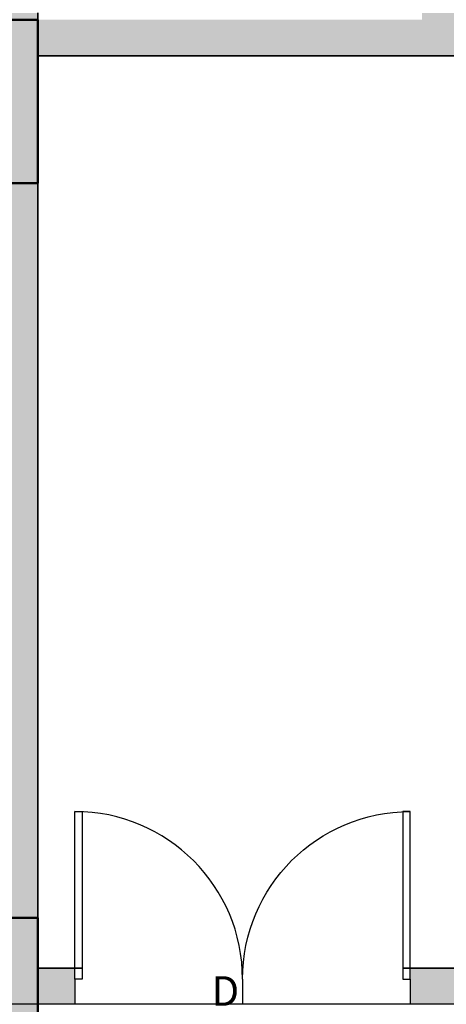
# Model space of a CAD drawing. Units: inches. Extents: x 1998 to 2588, y 1139 to 1977.
# Tile 122 of 134: x 2344 to 2397, y 1637 to 1760. Entities that reach past the tile are written whole.
import ezdxf

# ---------------------------------------------------------------- set-up
doc = ezdxf.new("R2010")
doc.units = ezdxf.units.IN
for name, color, linetype, lineweight in [('A-ANNO-DIMS', 2, 'Continuous', 18), ('A-COLS-PATT', 250, 'Continuous', 13), ('A-DOOR-IDEN', 7, 'Continuous', 18), ('A-WALL-PATT', 252, 'Continuous', 13), ('COLUMN', 10, 'Continuous', 50), ('DOOR', 52, 'Continuous', 25), ('WALL', 200, 'Continuous', 35)]:
    doc.layers.add(name, color=color, linetype=linetype, lineweight=lineweight)
doc.styles.get("Standard").update_dxf_attribs({"font": 'arial.ttf'})
doc.dimstyles.get("Standard").update_dxf_attribs({"dimtxt": 0.18, "dimasz": 0.18, "dimexe": 0.18, "dimexo": 0.0625, "dimgap": 0.09, "dimtad": 0, "dimtih": 1, "dimtoh": 1, "dimdec": 4, "dimzin": 0, "dimdsep": 46, "dimtxsty": 'Standard', "dimcen": 0.09, "dimadec": 0, "dimazin": 0, "dimtfac": 1, "dimtdec": 4, "dimtofl": 0, "dimtmove": 0, "dimatfit": 3, "dimfxl": 1, "dimtolj": 1, "dimtzin": 0, "dimarcsym": 0})

# ---------------------------------------------------------------- blocks, each defined once
blk = doc.blocks.new('*U2')
for p, q in [((0, 0), (0, -6)), ((40, 0), (40, -6))]:
    blk.add_line(p, q)
blk.add_lwpolyline([(0, 0), (0, 40), (1.75, 40), (1.75, 0)], close=True)
blk.add_arc((0, 0), 40, 0, 90)
blk = doc.blocks.new('*D30')
at = {"layer": 'A-ANNO-DIMS', "color": 0, "lineweight": -2, "transparency": 16777216}
for p, q in [((2407.91, 1636.73), (1997.84, 1636.73)), ((1998.02, 1636.55), (1998.02, 1615.91)), ((1998.02, 1594.91), (1998.02, 1615.55)), ((2407.91, 1594.73), (1997.84, 1594.73))]:
    blk.add_line(p, q, dxfattribs=at)
at = {"layer": 'A-ANNO-DIMS', "color": 0, "transparency": 16777216}
for points in [[(1997.99, 1636.55), (1998.05, 1636.55), (1998.02, 1636.73)], [(1997.99, 1594.91), (1998.05, 1594.91), (1998.02, 1594.73)]]:
    blk.add_solid(points, dxfattribs=at)
at = {"layer": 'Defpoints', "color": 0, "transparency": 16777216}
for p in [(1998.02, 1636.73), (2407.97, 1636.73), (2407.97, 1594.73)]:
    blk.add_point(p, dxfattribs=at)
at = {"layer": 'A-ANNO-DIMS', "color": 0, "transparency": 16777216, "insert": (1998.02, 1615.73), "char_height": 0.18, "attachment_point": 5}
blk.add_mtext('\\A1;42', dxfattribs=at)

msp = doc.modelspace()

# ---------------------------------------------------------------- hatches: boundary and pattern name
at = {"layer": 'A-COLS-PATT'}
h = msp.add_hatch(color=256, dxfattribs=at)
h.dxf.hatch_style = 1
h.paths.add_polyline_path([(2099.4125, 1888.7324), (2087.9729, 1888.7324), (2087.9729, 1868.3278), (2099.4125, 1868.3278)])
h.paths.add_polyline_path([(2234.4125, 1888.7324), (2222.9729, 1888.7324), (2222.9729, 1868.3278), (2234.4125, 1868.3278)])
h.paths.add_polyline_path([(2341.4729, 1886.637), (2330.0332, 1886.637), (2330.0332, 1866.2324), (2341.4729, 1866.2324)])
h.paths.add_polyline_path([(2507.8006, 1882.7324), (2487.396, 1882.7324), (2487.396, 1871.2927), (2507.8006, 1871.2927)])
h.paths.add_polyline_path([(2510.9729, 1766.672), (2490.5682, 1766.672), (2490.5682, 1755.2324), (2510.9729, 1755.2324)])
h.paths.add_polyline_path([(2345.9729, 1759.7324), (2334.5332, 1759.7324), (2334.5332, 1739.3278), (2345.9729, 1739.3278)])
h.paths.add_polyline_path([(2234.4125, 1774.3318), (2222.9729, 1774.3318), (2222.9729, 1753.9272), (2234.4125, 1753.9272)])
h.paths.add_polyline_path([(2099.4125, 1775.637), (2087.9729, 1775.637), (2087.9729, 1755.2324), (2099.4125, 1755.2324)])
h.paths.add_polyline_path([(2098.0956, 1593.7241), (2077.691, 1593.7241), (2077.691, 1582.2845), (2098.0956, 1582.2845)])
h.paths.add_polyline_path([(2227.4729, 1604.637), (2216.0332, 1604.637), (2216.0332, 1584.2324), (2227.4729, 1584.2324)])
h.paths.add_polyline_path([(2345.9729, 1647.5211), (2334.5332, 1647.5211), (2334.5332, 1627.1165), (2345.9729, 1627.1165)])
h.paths.add_polyline_path([(2522.3775, 1641.2324), (2501.9729, 1641.2324), (2501.9729, 1629.7927), (2522.3775, 1629.7927)])
h.paths.add_polyline_path([(2522.3775, 1480.7324), (2501.9729, 1480.7324), (2501.9729, 1469.2927), (2522.3775, 1469.2927)])
h.paths.add_polyline_path([(2345.9729, 1488.5616), (2334.5332, 1488.5616), (2334.5332, 1468.1569), (2345.9729, 1468.1569)])
h.paths.add_polyline_path([(2234.4125, 1486.137), (2227.4729, 1486.137), (2227.4729, 1465.7324), (2234.4125, 1465.7324)])
h.paths.add_polyline_path([(2227.4729, 1486.137), (2222.9729, 1486.137), (2222.9729, 1465.7324), (2227.4729, 1465.7324)])
h.paths.add_polyline_path([(2108.3775, 1470.2324), (2087.9729, 1470.2324), (2087.9729, 1458.7927), (2108.3775, 1458.7927)])
h.paths.add_polyline_path([(2096.9729, 1365.5012), (2087.9729, 1365.5012), (2087.9729, 1345.0966), (2096.9729, 1345.0966)])
h.paths.add_polyline_path([(2087.9729, 1365.5012), (2085.5332, 1365.5012), (2085.5332, 1345.0966), (2087.9729, 1345.0966)])
h.paths.add_polyline_path([(2234.4125, 1285.137), (2222.9729, 1285.137), (2222.9729, 1264.7324), (2234.4125, 1264.7324)])
h.paths.add_polyline_path([(2345.9729, 1285.137), (2334.5332, 1285.137), (2334.5332, 1264.7324), (2345.9729, 1264.7324)])
h.paths.add_polyline_path([(2503.1458, 1240.172), (2482.7412, 1240.172), (2482.7412, 1228.7324), (2503.1458, 1228.7324)])
h.paths.add_polyline_path([(2510.9729, 1369.172), (2490.5682, 1369.172), (2490.5682, 1357.7324), (2510.9729, 1357.7324)])
at = {"layer": 'A-WALL-PATT'}
h = msp.add_hatch(color=256, dxfattribs=at)
h.dxf.hatch_style = 1
h.paths.add_polyline_path([(2227.4729, 1911.2324), (2222.9729, 1911.2324), (2222.9729, 1888.7324), (2227.4729, 1888.7324)])
h.paths.add_polyline_path([(2236.4493, 1870.3636), (2236.4493, 1875.2324), (2234.4125, 1875.2324), (2234.4125, 1868.3278), (2227.4729, 1868.3278), (2227.4729, 1866.2324), (2236.4493, 1866.2324)])
h.paths.add_polyline_path([(2330.0332, 1875.2324), (2263.9907, 1875.2324), (2263.9907, 1866.2324), (2330.0332, 1866.2324)])
h.paths.add_polyline_path([(2345.9729, 1906.7324), (2393.9729, 1906.7324), (2393.9729, 1882.7324), (2345.9729, 1882.7324), (2345.9729, 1878.2324), (2393.9729, 1878.2324), (2398.4729, 1878.2324), (2398.4729, 1882.7324), (2398.4729, 1911.2324), (2345.9729, 1911.2324), (2341.4729, 1911.2324), (2341.4729, 1866.2324), (2341.4729, 1790.0412), (2345.9729, 1790.0412), (2345.9729, 1875.2324)])
h.paths.add_polyline_path([(2398.4729, 1878.2324), (2393.9729, 1878.2324), (2393.9729, 1798.2324), (2393.9729, 1793.7324), (2398.4729, 1793.7324)], flags=17)
h.paths.add_polyline_path([(2393.9729, 1798.2324), (2375.7311, 1798.2324, -0.00596797), (2375.7384, 1797.6146), (2375.7384, 1793.7324), (2393.9729, 1793.7324)], flags=17)
h.paths.add_polyline_path([(2349.8569, 1797.6146), (2349.8569, 1798.2324), (2345.9729, 1798.2324), (2345.9729, 1793.7324), (2349.8569, 1793.7324)], flags=17)
h.paths.add_polyline_path([(2398.4729, 1793.7324), (2393.9729, 1793.7324), (2393.9729, 1790.0412), (2398.4729, 1790.0412)], flags=17)
h.paths.add_polyline_path([(2527.4729, 1882.7324), (2507.8006, 1882.7324), (2507.8006, 1878.2324), (2518.4729, 1878.2324), (2518.4729, 1759.7324), (2510.9729, 1759.7324), (2510.9729, 1755.2324), (2527.4729, 1755.2324)])
h.paths.add_polyline_path([(2487.396, 1882.7324), (2398.4729, 1882.7324), (2398.4729, 1878.2324), (2487.396, 1878.2324)])
h.paths.add_polyline_path([(2490.5682, 1759.7324), (2345.9729, 1759.7324), (2345.9729, 1755.2324), (2490.5682, 1755.2324)])
h.paths.add_polyline_path([(2398.4729, 1760.5844), (2398.3914, 1760.5844), (2393.9729, 1760.5844), (2393.9729, 1759.7324), (2398.4729, 1759.7324)])
h.paths.add_polyline_path([(2334.5332, 1759.7324), (2234.4125, 1759.7324), (2234.4125, 1755.2324), (2334.5332, 1755.2324)])
h.paths.add_polyline_path([(2345.9729, 1760.5844), (2341.5543, 1760.5844), (2341.4729, 1760.5844), (2341.4729, 1759.7324), (2345.9729, 1759.7324)])
h.paths.add_polyline_path([(2222.9729, 1759.7324), (2221.7204, 1759.7324), (2221.7204, 1755.2324), (2222.9729, 1755.2324)])
h.paths.add_polyline_path([(2061.4729, 1702.7324), (2059.4729, 1702.7324), (2059.4729, 1584.2324), (2061.4729, 1584.2324)])
h.paths.add_polyline_path([(2061.4729, 1584.2324), (2059.4729, 1584.2324), (2059.4729, 1470.2324), (2061.4729, 1470.2324)])
h.paths.add_polyline_path([(2510.9729, 1469.2927), (2501.9729, 1469.2927), (2501.9729, 1369.172), (2510.9729, 1369.172)])
h.paths.add_polyline_path([(2227.4729, 1369.7324), (2227.4729, 1417.7324), (2221.4126, 1417.7324), (2221.4126, 1413.2324), (2222.9729, 1413.2324), (2222.9729, 1293.2324), (2222.9729, 1285.137), (2227.4729, 1285.137)])
h = msp.add_hatch(color=256, dxfattribs=at)
h.dxf.hatch_style = 1
h.paths.add_polyline_path([(2527.4729, 1362.2324), (2510.9729, 1362.2324), (2510.9729, 1357.7324), (2518.4729, 1357.7324), (2518.4729, 1237.7324), (2503.1458, 1237.7324), (2503.1458, 1228.7324), (2527.4729, 1228.7324)])
h.paths.add_polyline_path([(2490.5682, 1362.2324), (2398.4729, 1362.2324), (2398.4729, 1357.7324), (2490.5682, 1357.7324)])
h.paths.add_polyline_path([(2224.9729, 1264.7324), (2222.9729, 1264.7324), (2222.9729, 1232.4125), (2341.4729, 1232.4125), (2341.4729, 1234.4125), (2224.9729, 1234.4125)])
h.paths.add_polyline_path([(2334.5332, 1273.7324), (2264.7638, 1273.7324), (2264.7638, 1269.5611, -0.043659), (2264.3413, 1264.7324), (2334.5332, 1264.7324)])
h.paths.add_polyline_path([(2236.9551, 1273.7324), (2234.4125, 1273.7324), (2234.4125, 1264.7324), (2236.9551, 1264.7324), (2236.9551, 1269.5611)])
h.paths.add_polyline_path([(2222.9729, 1293.2324), (2096.9729, 1293.2324), (2096.9729, 1345.0966), (2087.9729, 1345.0966), (2087.9729, 1284.2324), (2222.9729, 1284.2324), (2222.9729, 1285.137)])
h.paths.add_polyline_path([(2096.9729, 1458.7927), (2087.9729, 1458.7927), (2087.9729, 1417.7324), (2087.9729, 1413.2324), (2096.9729, 1413.2324), (2096.9729, 1417.7324)])
h.paths.add_polyline_path([(2096.9729, 1413.2324), (2087.9729, 1413.2324), (2087.9729, 1365.5012), (2096.9729, 1365.5012), (2096.9729, 1369.3358)])
h.paths.add_polyline_path([(2186.2943, 1417.7324), (2138.6074, 1417.7324), (2096.9729, 1417.7324), (2096.9729, 1413.2324), (2138.6074, 1413.2324), (2186.2943, 1413.2324)])
h.paths.add_polyline_path([(2181.4729, 1465.7324), (2176.9729, 1465.7324), (2176.9729, 1451.6434), (2181.4729, 1451.6434)])
h.paths.add_polyline_path([(2181.4729, 1422.1664), (2176.9729, 1422.1664), (2176.9729, 1417.7324), (2181.4729, 1417.7324)])
h.paths.add_polyline_path([(2063.9729, 1465.7324), (2087.9729, 1465.7324), (2087.9729, 1470.2324), (2059.4729, 1470.2324), (2059.4729, 1413.2324), (2087.9729, 1413.2324), (2087.9729, 1417.7324), (2063.9729, 1417.7324)])
h.paths.add_polyline_path([(2181.4729, 1755.2324), (2176.9729, 1755.2324), (2176.9729, 1748.6798), (2177.0513, 1748.6798), (2181.4729, 1748.6798)])
h.paths.add_polyline_path([(2227.4729, 1707.2324), (2220.4647, 1707.2324), (2220.4647, 1702.7324), (2222.9729, 1702.7324), (2222.9729, 1604.637), (2227.4729, 1604.637)])
h.paths.add_polyline_path([(2114.9729, 1702.7324), (2105.9729, 1702.7324), (2105.9729, 1628.4781, -0.0318759), (2110.1012, 1628.7416), (2114.9729, 1628.7416)])
h.paths.add_polyline_path([(2345.9729, 1739.3278), (2341.4729, 1739.3278), (2341.4729, 1647.5211), (2345.9729, 1647.5211)])
h.paths.add_polyline_path([(2350.6273, 1641.2324), (2345.9729, 1641.2324), (2345.9729, 1636.7324), (2350.6273, 1636.7324), (2350.6273, 1639.8729)])
h.paths.add_polyline_path([(2501.9729, 1641.2324), (2407.9729, 1641.2324), (2392.5005, 1641.2324), (2392.5005, 1639.8729), (2392.5005, 1636.7324), (2501.9729, 1636.7324)])
h.paths.add_polyline_path([(2510.9729, 1755.2324), (2501.9729, 1755.2324), (2501.9729, 1641.2324), (2510.9729, 1641.2324)])
h.paths.add_polyline_path([(2549.1786, 1641.2324), (2522.3775, 1641.2324), (2522.3775, 1636.7324), (2540.1786, 1636.7324), (2540.1786, 1480.7324), (2522.3775, 1480.7324), (2522.3775, 1476.2324), (2549.1786, 1476.2324)])
h.paths.add_polyline_path([(2498.1786, 1594.7324), (2407.9729, 1594.7324), (2407.9729, 1585.7324), (2416.9729, 1585.7324), (2489.1786, 1585.7324), (2489.1786, 1531.7324), (2416.9729, 1531.7324), (2407.9729, 1531.7324), (2407.9729, 1522.7324), (2498.1786, 1522.7324)])
h.paths.add_polyline_path([(2351.6437, 1480.7324), (2345.9729, 1480.7324), (2345.9729, 1476.2324), (2351.6437, 1476.2324), (2351.6437, 1477.5919)])
h.paths.add_polyline_path([(2501.9729, 1480.7324), (2498.1786, 1480.7324), (2407.9729, 1480.7324), (2393.5168, 1480.7324), (2393.5168, 1477.5919), (2393.5168, 1476.2324), (2501.9729, 1476.2324)])

# ---------------------------------------------------------------- linework, layer by layer
at = {"layer": 'COLUMN'}
for points in [[(2334.5332, 1759.7324), (2345.9729, 1759.7324), (2345.9729, 1739.3278), (2334.5332, 1739.3278)], [(2334.5332, 1647.5211), (2345.9729, 1647.5211), (2345.9729, 1627.1165), (2334.5332, 1627.1165)]]:
    msp.add_lwpolyline(points, close=True, dxfattribs=at)
at = {"layer": 'WALL'}
for p, q in [((2345.9729, 1755.2324), (2345.9729, 1760.5844)), ((2345.9729, 1755.2324), (2527.4729, 1755.2324)), ((2345.9729, 1755.2324), (2345.9729, 1588.7324)), ((2345.9729, 1755.2324), (2501.9729, 1755.2324)), ((2351.5433, 1641.2324), (2345.9729, 1641.2324)), ((2371.6081, 1641.2324), (2371.5197, 1641.2324)), ((2501.9729, 1641.2324), (2391.5845, 1641.2324))]:
    msp.add_line(p, q, dxfattribs=at)

# ---------------------------------------------------------------- block references
at = {"layer": 'DOOR', "yscale": 0.5234138920659225, "zscale": 0.5234138920659225}
for p, xscale in [((2350.6273, 1639.8729), 0.5234138920659225), ((2392.5005, 1639.8729), -0.5234138920659225)]:
    msp.add_blockref('*U2', p, dxfattribs=dict(at, xscale=xscale))

# ---------------------------------------------------------------- texts
at = {"layer": 'A-DOOR-IDEN', "insert": (2367.677, 1640.2432), "char_height": 3.6988, "attachment_point": 1}
msp.add_mtext_dynamic_manual_height_columns('D', width=110.572713, gutter_width=18.4938, heights=[0], dxfattribs=at)

# ---------------------------------------------------------------- dimensions: what is measured, and where the dimension line sits
at = {"layer": 'A-ANNO-DIMS'}
dim = msp.add_linear_dim(base=(1998.0229, 1636.7324), p1=(2407.9729, 1594.7324), p2=(2407.9729, 1636.7324), angle=90, dimstyle='Standard', override={"dimdec": 0, "dimlfac": 1, "dimrnd": 0, "dimzin": 0, "dimdsep": 46, "dimlunit": 2}, dxfattribs=at)
dim.commit()
dim.dimension.update_dxf_attribs({"geometry": '*D30', "text_midpoint": (1998.0229, 1615.7324)})

doc.saveas('drawing.dxf')
